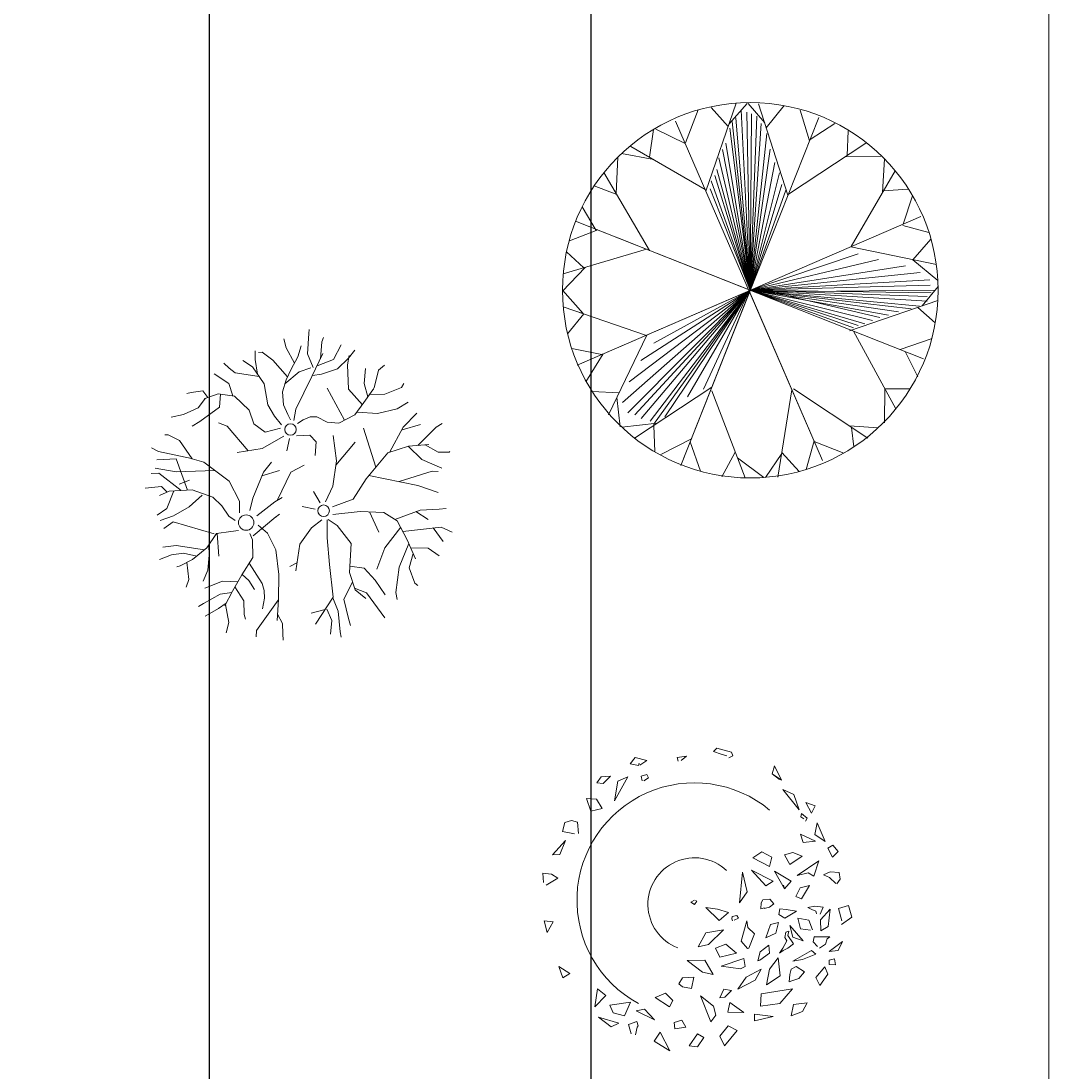
# Model space of a CAD drawing. Units: inches. Extents: x 8049 to 8459, y 820 to 1350.
# Tile 14 of 25: x 8170 to 8197, y 879 to 906. Entities that reach past the tile are written whole.
import ezdxf

# ---------------------------------------------------------------- set-up
doc = ezdxf.new("R2010")
doc.units = ezdxf.units.IN
doc.header["$MEASUREMENT"] = 0
for name, color, linetype, lineweight in [('A-ANNO-DIMS', 2, 'Continuous', 18), ('L-PLNT-BEDS', 94, 'Continuous', 18), ('zelen', 69, 'Continuous', 13)]:
    doc.layers.add(name, color=color, linetype=linetype, lineweight=lineweight)
doc.styles.get("Standard").update_dxf_attribs({"font": 'arial.ttf'})
doc.dimstyles.get("Standard").update_dxf_attribs({"dimtxt": 0.18, "dimasz": 0.18, "dimexe": 0.18, "dimexo": 0.0625, "dimgap": 0.09, "dimtad": 0, "dimtih": 1, "dimtoh": 1, "dimdec": 4, "dimzin": 0, "dimdsep": 46, "dimtxsty": 'Standard', "dimcen": 0.09, "dimadec": 0, "dimazin": 0, "dimtfac": 1, "dimtdec": 4, "dimtofl": 0, "dimtmove": 0, "dimatfit": 3, "dimfxl": 1, "dimtolj": 1, "dimtzin": 0, "dimarcsym": 0})

# ---------------------------------------------------------------- blocks, each defined once
blk = doc.blocks.new('T40C')
for p, q in [((-0.1219, 0.4263), (-0.1133, 0.5002)), ((-0.0016, 0.4444), (-0.055, 0.5069)), ((-0.0016, 0.0138), (-0.0016, 0.5115)), ((-0.0016, 0.5115), (-0.0016, -0.4769)), ((-0.0016, 0.4364), (0.0585, 0.5048)), ((0.1041, 0.4402), (0.0754, 0.5038)), ((-0.0047, 0.2984), (-0.1711, 0.4799)), ((-0.0016, 0.2889), (0.1386, 0.4896)), ((0.0979, 0.4313), (0.1806, 0.4751)), ((0.2217, 0.4068), (0.1848, 0.4759)), ((-0.2, 0.2178), (-0.2513, 0.4459)), ((-0.2374, 0.3843), (-0.221, 0.4586)), ((-0.1327, 0.438), (-0.2166, 0.4607)), ((0.2091, 0.2244), (0.2252, 0.4573)), ((-0.0016, 0.0138), (0.1054, 0.4378)), ((-0.0016, 0.0138), (0.1166, 0.4328)), ((0.0011, 0.0164), (0.1417, 0.4349)), ((0.0011, 0.0164), (0.1801, 0.4343)), ((0.0011, 0.0164), (0.161, 0.432)), ((0.2208, 0.3933), (0.2879, 0.4166)), ((-0.3045, 0.3219), (-0.313, 0.3998)), ((-0.2369, 0.3817), (-0.2976, 0.4118)), ((-0.0016, 0.0138), (0.2033, 0.4135)), ((-0.0016, 0.0138), (0.0852, 0.4075)), ((0.2979, 0.3132), (0.3134, 0.399)), ((0.3508, 0.3661), (-0.3487, -0.3333)), ((0.0011, 0.0164), (-0.3443, 0.3618)), ((-0.3443, 0.3618), (0.3464, -0.329)), ((0.0011, 0.0164), (0.3508, 0.3661)), ((-0.0016, 0.0138), (0.2072, 0.3567)), ((0.0011, 0.0164), (0.0491, 0.3369)), ((-0.3055, 0.3229), (-0.3893, 0.3231)), ((0.3008, 0.3162), (0.3801, 0.3306)), ((-0.3838, 0.2523), (-0.4084, 0.2975)), ((-0.0016, 0.0138), (0.1989, 0.2926)), ((0.0011, 0.0164), (0.0175, 0.3021)), ((0.3847, 0.2335), (0.4047, 0.2984)), ((-0.377, 0.2509), (-0.4492, 0.2275)), ((-0.2034, 0.2144), (-0.4335, 0.2627)), ((-0.0016, 0.0138), (0.1836, 0.2378)), ((0.2092, 0.2254), (0.4418, 0.2362)), ((0.3861, 0.2336), (0.4597, 0.1963)), ((0.3915, 0.2339), (0.3982, 0.2342)), ((-0.4278, 0.1246), (-0.4601, 0.209)), ((0.4263, 0.1181), (0.4586, 0.1989)), ((-0.2946, 0.0138), (-0.4744, 0.1635)), ((0.2937, 0.0138), (0.4738, 0.1555)), ((-0.4281, 0.1249), (-0.4899, 0.1006)), ((0.4291, 0.1204), (0.4873, 0.0978)), ((-0.4418, 0.0138), (-0.4967, 0.0634)), ((0.4315, 0.0138), (0.491, 0.0679)), ((-0.4277, 0.0138), (-0.4952, -0.0443)), ((0.4953, 0.0138), (-0.4939, 0.0138)), ((-0.2846, 0.0167), (-0.4721, -0.1432)), ((-0.0016, 0.0138), (-0.4477, -0.1559)), ((-0.0016, 0.0138), (-0.4464, -0.1312)), ((-0.0016, 0.0138), (-0.4422, -0.1429)), ((-0.0016, 0.0138), (-0.4379, -0.1735)), ((-0.0016, 0.0138), (-0.4328, -0.1117)), ((-0.0016, 0.0138), (-0.4324, -0.1862)), ((-0.4324, -0.1862), (-0.0016, 0.0138)), ((-0.0016, 0.0138), (-0.4146, -0.0968)), ((-0.0016, 0.0138), (-0.4013, -0.1946)), ((-0.0016, 0.0138), (-0.3864, -0.0775)), ((-0.0016, 0.0138), (-0.3647, -0.0593)), ((-0.0016, 0.0138), (-0.3588, -0.1967)), ((-0.0016, 0.0138), (-0.3309, -0.0302)), ((-0.0016, 0.0138), (-0.3156, -0.0151)), ((-0.0016, 0.0138), (-0.3007, -0.0042)), ((-0.0016, 0.0138), (-0.2917, 0.0059)), ((-0.0016, 0.0138), (-0.2861, -0.1863)), ((-0.0016, 0.0138), (-0.2311, -0.181)), ((-0.0016, 0.0138), (-0.0528, -0.0021)), ((-0.0016, 0.0138), (-0.0528, -0.0021)), ((-0.0016, 0.0138), (0.0011, 0.0164)), ((-0.0016, 0.0138), (0.4953, 0.0138)), ((-0.0016, 0.0138), (0.0088, -0.2669)), ((-0.0016, 0.0138), (0.0243, -0.2768)), ((-0.0016, 0.0138), (0.0408, -0.3033)), ((-0.0016, 0.0138), (0.0625, -0.3241)), ((-0.0016, 0.0138), (0.0872, -0.3518)), ((-0.0016, 0.0138), (0.1104, -0.3878)), ((-0.0016, 0.0138), (0.1339, -0.4064)), ((-0.0016, 0.0138), (0.1521, -0.4202)), ((-0.0016, 0.0138), (0.1669, -0.4211)), ((-0.0016, 0.0138), (0.1801, -0.4202)), ((-0.0016, 0.0138), (0.1959, -0.4202)), ((-0.0016, 0.0138), (0.2013, -0.3955)), ((-0.0016, 0.0138), (0.2072, -0.3832)), ((-0.0016, 0.0138), (0.2062, -0.3647)), ((-0.0016, 0.0138), (0.2018, -0.3233)), ((-0.0016, 0.0138), (0.2038, -0.3052)), ((-0.0016, 0.0138), (0.2044, -0.2809)), ((-0.0016, 0.0138), (0.1983, -0.2504)), ((-0.0016, 0.0138), (0.197, -0.2334)), ((-0.0016, 0.0138), (0.2007, -0.2173)), ((-0.0016, 0.0138), (0.1959, -0.1959)), ((0.285, 0.0138), (0.4722, -0.133)), ((0.2917, 0.0138), (0.3747, 0.0138)), ((0.4349, 0.0169), (0.4927, -0.0276)), ((-0.0528, -0.0021), (-0.4551, -0.1664)), ((-0.0528, -0.0021), (-0.3463, -0.045)), ((-0.4294, -0.1068), (-0.4874, -0.0863)), ((0.4191, -0.0914), (0.4833, -0.0909)), ((0.4217, -0.0934), (0.4533, -0.184)), ((-0.4387, -0.1147), (-0.459, -0.1779)), ((-0.3712, -0.2192), (-0.4529, -0.1923)), ((-0.2066, -0.1906), (-0.4335, -0.23)), ((-0.2067, -0.1914), (-0.2414, -0.4204)), ((0.2042, -0.1867), (0.2149, -0.4325)), ((0.2071, -0.1897), (0.4318, -0.2236)), ((-0.3712, -0.2192), (-0.3953, -0.2872)), ((0.3628, -0.2132), (0.4476, -0.1967)), ((0.3755, -0.2151), (0.3928, -0.2871)), ((-0.0016, -0.2596), (-0.1424, -0.4599)), ((-0.0016, -0.2565), (0.16, -0.4525)), ((-0.3126, -0.2938), (-0.3837, -0.3016)), ((-0.3124, -0.2971), (-0.3082, -0.3761)), ((0.3007, -0.2833), (0.3874, -0.2905)), ((0.3008, -0.2851), (0.3017, -0.3787)), ((-0.2322, -0.3601), (-0.2902, -0.3882)), ((-0.2315, -0.3548), (-0.2033, -0.4394)), ((0.2123, -0.3741), (0.1875, -0.442)), ((0.212, -0.3667), (0.2724, -0.3967)), ((-0.1046, -0.4061), (-0.1917, -0.4425)), ((-0.1086, -0.4118), (-0.0869, -0.4727)), ((-0.0016, -0.4144), (-0.047, -0.4779)), ((-0.0016, -0.4109), (0.0515, -0.477)), ((0.1172, -0.4006), (0.0947, -0.4728)), ((0.1259, -0.4112), (0.1857, -0.4428))]:
    blk.add_line(p, q)
blk.add_circle((-0.0016, 0.0138), 0.496)
blk = doc.blocks.new('z_115')
for p, q in [((-18.8, 436.5), (-14.5, 500.6)), ((-14.5, 500.6), (-13.6, 513.4)), ((-86.5, 455.8), (-94.6, 483.9)), ((22, 420.7), (26.8, 474.3)), ((26.8, 474.3), (31.7, 488.4)), ((-184.5, 418.6), (-185.4, 446.1)), ((-162.6, 441.7), (-174.6, 440.4)), ((-129.1, 416.7), (-162.6, 441.7)), ((-60.7, 407), (-86.5, 455.8)), ((-49.9, 426.9), (-39.4, 462.2)), ((-1.4, 393.4), (-18.8, 436.5)), ((-4.9, 364.2), (29.9, 437.2)), ((63.4, 418.3), (87.8, 464.7)), ((111.2, 422.4), (130.6, 448.1)), ((-267.7, 390.7), (-284, 406.4)), ((-193.4, 394.9), (-223.9, 415.7)), ((-177.4, 372), (-184.5, 418.6)), ((-82.4, 363.5), (-129.1, 416.7)), ((-71.1, 387.5), (-49.9, 426.9)), ((11.4, 398.3), (63.4, 418.3)), ((76.1, 388.5), (111.2, 422.4)), ((107.5, 401.6), (113, 430.8)), ((111.2, 324.1), (107.5, 401.6)), ((205.4, 384.6), (225.1, 401)), ((-268.3, 342.4), (-315.1, 373.1)), ((-248.2, 376.3), (-267.7, 390.7)), ((-172.4, 364.7), (-248.2, 376.3)), ((-156.2, 341.4), (-193.4, 394.9)), ((-90.7, 340.9), (-45.9, 379.2)), ((-86.9, 353.9), (-71.1, 387.5)), ((-45.9, 379.2), (-8.3, 392.3)), ((-3.1, 368.1), (25.6, 372.2)), ((25.6, 372.2), (76.1, 388.5)), ((160.2, 342.1), (164.2, 389.5)), ((192.5, 328.6), (205.4, 384.6)), ((-255.3, 302.8), (-268.3, 342.4)), ((-144.5, 275.1), (-156.2, 341.4)), ((-98.3, 315.8), (-86.9, 353.9)), ((-55.7, 261), (-4.9, 364.2)), ((171.8, 299.6), (160.2, 342.1)), ((278.7, 329.2), (286.1, 342.4)), ((-387.5, 313.5), (-401, 310.3)), ((-350.5, 319.6), (-387.5, 313.5)), ((-335.4, 298.2), (-350.5, 319.6)), ((-302.1, 309.7), (-346.5, 294.3)), ((-250.4, 302), (-302.1, 309.7)), ((-294.4, 308.5), (-298.1, 267.8)), ((-203.9, 258.1), (-250.4, 302)), ((-95.5, 274.5), (-98.3, 315.8)), ((97.9, 225.7), (42.8, 327.6)), ((155.1, 275.2), (111.2, 324.1)), ((159.9, 282.2), (182.3, 314.8)), ((177.4, 307.7), (226.4, 308.4)), ((182.3, 314.8), (191.3, 327)), ((226.4, 308.4), (278.7, 329.2)), ((-342.4, 295.8), (-365.9, 265.5)), ((-298.1, 267.8), (-360.4, 221.6)), ((-124.1, 238.9), (-144.5, 275.1)), ((-81.6, 243.7), (-95.5, 274.5)), ((131.2, 242.8), (159.9, 282.2)), ((264.6, 262), (300, 283.1)), ((-412.1, 244), (-450.9, 235.7)), ((-365.9, 265.5), (-412.1, 244)), ((-189.7, 214.3), (-203.9, 258.1)), ((-101.3, 211.6), (-124.1, 238.9)), ((-72.6, 227.6), (-81.6, 243.7)), ((-61.9, 224.8), (-55.7, 261)), ((-33, 226.8), (-11.1, 237)), ((-11.1, 237), (10.2, 237)), ((10.2, 237), (43.7, 220)), ((80.7, 216.8), (131.2, 242.8)), ((137.8, 251.8), (202.7, 247.6)), ((202.7, 247.6), (264.6, 262)), ((284, 204.3), (327.4, 248.5)), ((-360.4, 221.6), (-384.1, 206.6)), ((-273.2, 207.5), (-301.5, 217.8)), ((-206.8, 129.4), (-273.2, 207.5)), ((-152.8, 187.7), (-189.7, 214.3)), ((-104.5, 200.6), (-152.8, 187.7)), ((-50.6, 215.3), (-33, 226.8)), ((43.7, 220), (80.7, 216.8)), ((197.6, 76.9), (158.9, 201.1)), ((241, 124.1), (284, 204.3)), ((281.2, 196), (338.5, 212.3)), ((330.6, 146), (388.4, 203.7)), ((388.4, 203.7), (407.5, 215.5)), ((-461.1, 179.4), (-470.9, 180)), ((-424.4, 162.1), (-461.1, 179.4)), ((-94.2, 175.3), (-163.2, 136.1)), ((-75.7, 168.1), (-84.7, 128.4)), ((-53.8, 176.8), (-11.4, 178.7)), ((-11.4, 178.7), (8, 157.9)), ((73, 96.7), (62.2, 177.8)), ((-491.6, 126.5), (-513.4, 138)), ((-384.4, 104), (-424.4, 162.1)), ((-163.2, 136.1), (-242.4, 123.9)), ((8, 157.9), (5.5, 114)), ((71.1, 83.3), (132.4, 156.9)), ((235.6, 122.3), (301.5, 143.8)), ((299.9, 143.7), (343.1, 101.2)), ((301.5, 143.8), (365.3, 148.6)), ((354.1, 147.8), (394.5, 124.9)), ((-435.2, 103.8), (-496.2, 99.9)), ((-387.1, 104.7), (-491.6, 126.5)), ((-399.6, 4.6), (-435.2, 103.8)), ((-347.4, 93.2), (-391.5, 106)), ((166.9, 40.4), (235.6, 122.3)), ((343.1, 101.2), (406.3, 74)), ((394.5, 124.9), (429.4, 124.9)), ((429.4, 124.9), (432.1, 126.5)), ((-434.9, 62.5), (-501.7, 74)), ((-312.8, 66.9), (-434.9, 62.5)), ((-267.7, 32.7), (-347.4, 93.2)), ((-158.6, 61.2), (-132.7, 93.2)), ((-71.8, 61.2), (-29.6, 83.9)), ((61.6, 17), (73, 96.7)), ((-490, 58), (-515, 57)), ((-419.6, 3.5), (-490, 58)), ((-392.7, 35.9), (-425.7, 23.1)), ((-192.8, -21.5), (-158.6, 61.2)), ((-163.3, 49.8), (-107.5, 66.3)), ((-115.7, -28.8), (-71.8, 61.2)), ((126, -24.3), (166.9, 40.4)), ((175.7, 50.8), (330.2, 19.2)), ((271, 31.3), (376.4, 64.1)), ((376.4, 64.1), (395.5, 63.1)), ((-481.7, 16.3), (-533.5, 10.6)), ((-457.4, 1.3), (-488.2, -12.8)), ((-464, -1.8), (-481.7, 16.3)), ((-442.9, 2.1), (-465.1, -53.8)), ((-385, 5.4), (-457.4, 1.3)), ((-319.1, -17.9), (-385, 5.4)), ((-235, -30.4), (-267.7, 32.7)), ((20.8, -35.8), (0, 0)), ((38.1, -32.9), (61.6, 17)), ((330.2, 19.2), (395.5, -3.5)), ((-353.3, -11.5), (-394.5, -49)), ((-290.4, -45.2), (-319.1, -17.9)), ((-234.8, -67.7), (-235, -30.4)), ((-201.7, -60.6), (-192.8, -21.5)), ((-179.5, -77.2), (-122.3, -32.7)), ((-122.3, -32.7), (-99.2, -18.9)), ((60.5, -49.2), (126, -24.3)), ((-465.1, -53.8), (-495.6, -74.6)), ((-394.5, -49), (-444.1, -77.2)), ((-268, -78.8), (-290.4, -45.2)), ((5.5, -56.2), (-36, -48)), ((61.1, -73.3), (147.5, -63.4)), ((147.5, -63.4), (222.4, -66.3)), ((177.6, -64.6), (207.3, -129.1)), ((222.4, -66.3), (265.5, -93.5)), ((258.1, -88.8), (337.6, -59.6)), ((324, -63.1), (363.7, -88.7)), ((337.6, -59.6), (397.9, -55.7)), ((397.9, -55.7), (420.7, -53.5)), ((-444.1, -77.2), (-486, -91.9)), ((-444.4, -96.7), (-474, -117.5)), ((-314.6, -134.2), (-444.4, -96.7)), ((-248.3, -92.1), (-268, -78.8)), ((-119.3, -80.2), (-191.3, -140.3)), ((-108.1, -71.7), (-122, -82.3)), ((25.9, -89.8), (-6.8, -115.6)), ((43, -89.7), (43.4, -146.7)), ((46.4, -88.4), (74.8, -107.6)), ((265.5, -93.5), (296.9, -152.8)), ((-262.1, -127.1), (-307.1, -133.2)), ((-305.3, -133), (-300.3, -204.7)), ((-237.6, -123.2), (-262.1, -127.1)), ((-202.1, -132.9), (-193.1, -153.7)), ((-175.4, -107.1), (-146.3, -132.3)), ((-146.3, -132.3), (-119.5, -185.4)), ((-6.8, -115.6), (-43.1, -167.5)), ((74.8, -107.6), (119.8, -164.9)), ((276.2, -113.6), (225.5, -179)), ((282.9, -126.4), (404.4, -113.1)), ((379.5, -115), (410.6, -158.2)), ((404.4, -113.1), (439.8, -128.7)), ((-307.1, -133.2), (-338.5, -178.7)), ((-193.1, -153.7), (-192.8, -209.8)), ((43.4, -146.7), (50.5, -231.2)), ((119.8, -164.9), (114, -256.5)), ((302.2, -165.1), (271.3, -239.9)), ((296.9, -152.8), (323.1, -213.9)), ((-435.8, -171.7), (-477.7, -176.8)), ((-412.1, -196), (-449.7, -200.8)), ((-345.7, -184.7), (-435.8, -171.7)), ((-370.3, -205.2), (-412.1, -196)), ((-338.5, -178.7), (-383.2, -215.9)), ((-331.8, -169), (-330.2, -201.8)), ((-119.5, -185.4), (-109.6, -262.9)), ((-43.1, -167.5), (-56.4, -251.1)), ((225.5, -179), (200.5, -246.3)), ((315.6, -196.4), (303.1, -242.1)), ((308, -178.8), (363.4, -180)), ((363.4, -180), (398.2, -204)), ((-449.7, -200.8), (-487.6, -215.5)), ((-383.2, -215.9), (-422.9, -235.4)), ((-401, -224.6), (-395.5, -279.3)), ((-330.2, -201.8), (-335.4, -249.2)), ((-192.8, -209.8), (-226.7, -263.9)), ((-203.8, -227.4), (-162.3, -292.1)), ((-52.5, -226.5), (-74.8, -238)), ((50.5, -231.2), (62.2, -335)), ((-422.9, -235.4), (-433, -238.6)), ((-335.4, -249.2), (-349.3, -284.7)), ((-226.7, -263.9), (-257.2, -316.1)), ((-226, -262.8), (-205.1, -282.2)), ((-109.6, -262.9), (-111.5, -342.4)), ((114, -256.5), (131.8, -311.6)), ((115.2, -236.5), (160.5, -243.1)), ((160.5, -243.1), (195.3, -280.9)), ((271.3, -239.9), (260.9, -320.6)), ((303.1, -242.1), (321.2, -290.5)), ((-395.5, -279.3), (-403.2, -303.6)), ((-288.3, -284.4), (-344.7, -307.1)), ((-239.6, -286.1), (-288.3, -284.4)), ((-205.1, -282.2), (-187, -310.7)), ((-162.3, -292.1), (-156.8, -314.2)), ((123.9, -287.2), (95.8, -341.4)), ((195.3, -280.9), (227, -327.3)), ((321.2, -290.5), (330.8, -298.2)), ((-296, -325.4), (-348.3, -355.5)), ((-259.3, -320.1), (-296, -325.4)), ((-257.2, -316.1), (-280.9, -362.2)), ((-249.1, -302.2), (-221.1, -346.5)), ((-156.8, -314.2), (-155.8, -338.2)), ((130.2, -306.7), (167.9, -320.9)), ((131.8, -311.6), (166, -339.5)), ((167.9, -320.9), (225.5, -401)), ((260.9, -320.6), (264.9, -343)), ((-348.3, -355.5), (-364.4, -365.1)), ((-276.6, -353.8), (-301.5, -371.5)), ((-278.8, -358.2), (-268.6, -415.4)), ((-221.1, -346.5), (-219.9, -389.8)), ((-111.6, -344.9), (-180.5, -441.3)), ((-155.8, -338.2), (-161.7, -371.8)), ((-111.5, -342.4), (-115.5, -409.6)), ((62.2, -335), (6.5, -421.2)), ((61.1, -336.8), (77.6, -379.5)), ((95.8, -341.4), (111.2, -402.9)), ((-301.5, -371.5), (-343.7, -395.5)), ((-219.9, -389.8), (-215.6, -404.5)), ((-114.3, -389.5), (-97.9, -418.6)), ((36.7, -374.4), (-8, -385.6)), ((42.5, -373), (58.5, -409.6)), ((77.6, -379.5), (84.1, -444.9)), ((-268.6, -415.4), (-277.2, -447.7)), ((-97.9, -418.6), (-97.3, -451.3)), ((58.5, -409.6), (53.6, -452.5)), ((111.2, -402.9), (117.7, -425.3)), ((-180.5, -441.3), (-181.7, -460.9)), ((-97.3, -451.3), (-96.4, -471.1)), ((84.1, -444.9), (87.2, -462.2))]:
    blk.add_line(p, q)
for centre, radius in [((-73, 196.5), 18.1), ((31.9, -61.1), 18.3), ((-213.5, -98.7), 24.4)]:
    blk.add_circle(centre, radius)
blk = doc.blocks.new('z_66')
for p, q in [((83.2, 488.9), (72.7, 477.7)), ((72.7, 477.7), (96.4, 469.7)), ((129.8, 476.2), (83.2, 488.9)), ((96.4, 469.7), (114.5, 463.9)), ((134, 464.6), (129.8, 476.2)), ((-176.4, 458.5), (-191.7, 438.6)), ((-191.7, 438.6), (-165.6, 433.5)), ((-139.2, 449.4), (-176.4, 458.5)), ((-165.6, 433.5), (-163.6, 441.1)), ((-165.6, 433.5), (-165.6, 433.5)), ((-161.1, 434.6), (-139.2, 449.4)), ((-13.6, 463.6), (-42.5, 459.2)), ((-42.5, 459.2), (-39.3, 446.9)), ((-30.3, 449.4), (-13.6, 463.6)), ((114.5, 463.9), (114.5, 463.9)), ((120.4, 457.8), (134, 464.6)), ((-254, 399.9), (-283.6, 397.7)), ((-272.8, 380.7), (-254, 399.9)), ((-138.9, 404.9), (-156.9, 400.2)), ((-156.9, 400.2), (-153.8, 385.4)), ((-133.3, 394.8), (-138.9, 404.9)), ((265.2, 432.1), (258.2, 407.5)), ((258.2, 407.5), (287.4, 387.2)), ((258.2, 407.5), (281.9, 388.6)), ((287.4, 387.2), (265.2, 432.1)), ((-283.6, 397.7), (-297.2, 378.2)), ((-297.2, 378.2), (-277.7, 376)), ((-277.7, 376), (-272.8, 380.7)), ((-241.9, 321.7), (-199.1, 397.3)), ((-231.4, 383.6), (-241.9, 321.7)), ((-199.1, 397.3), (-231.4, 383.6)), ((-148.6, 384.7), (-133.3, 394.8)), ((281.9, 388.6), (281.9, 388.6)), ((344.2, 293.1), (292, 357.2)), ((292, 357.2), (326.8, 341.2)), ((326.8, 341.2), (344.2, 293.1)), ((-330.3, 328.9), (-298.6, 327.1)), ((-316, 288.8), (-330.3, 328.9)), ((-298.6, 327.1), (-280.8, 297.1)), ((383.1, 281.9), (364.4, 316.3)), ((364.4, 316.3), (394.6, 305.1)), ((394.6, 305.1), (383.1, 281.9)), ((-280.8, 297.1), (-316, 288.8)), ((350.8, 280.8), (348.7, 270.3)), ((348.7, 270.3), (358.8, 264.5)), ((369.2, 266.7), (350.8, 280.8)), ((363.3, 256.6), (369.2, 266.7)), ((-399.2, 252.6), (-405.8, 224)), ((-377.9, 259.1), (-399.2, 252.6)), ((-358.4, 254), (-377.9, 259.1)), ((-356, 217.5), (-358.4, 254)), ((358.8, 264.5), (358.8, 264.5)), ((400.9, 251.9), (393.9, 214.6)), ((426.6, 192.2), (400.9, 251.9)), ((-405.8, 224), (-368.2, 216.4)), ((-368.2, 216.4), (-368.2, 216.4)), ((348, 215.7), (356, 188.9)), ((395.3, 193.2), (348, 215.7)), ((393.9, 214.6), (426.6, 192.2)), ((-396.4, 196.1), (-438.1, 150.2)), ((-414.8, 150.9), (-396.4, 196.1)), ((356, 188.9), (395.3, 193.2)), ((450, 180.6), (434.3, 171.2)), ((434.3, 171.2), (449.6, 142.6)), ((467.7, 160.3), (450, 180.6)), ((-438.1, 150.2), (-414.8, 150.9)), ((225.2, 159.9), (197, 140.8)), ((197, 140.8), (249.5, 113.6)), ((256.8, 142.6), (225.2, 159.9)), ((249.5, 113.6), (256.8, 142.6)), ((323.6, 157.8), (297.5, 149.8)), ((297.5, 149.8), (314.6, 119.4)), ((314.6, 119.4), (352.9, 145.5)), ((352.9, 145.5), (323.6, 157.8)), ((449.6, 142.6), (467.7, 160.3)), ((193.1, 101.3), (238, 52.1)), ((261.7, 66.6), (193.1, 101.3)), ((336.9, 84.3), (405.8, 131.7)), ((405.8, 131.7), (389.8, 82.1)), ((-468.4, 91.6), (-466.3, 62.6)), ((-441.6, 89), (-468.4, 91.6)), ((-458.3, 53.9), (-421.1, 76)), ((-421.1, 76), (-441.6, 89)), ((164.3, 94.8), (154.2, -2.2)), ((178.9, 33.3), (164.3, 94.8)), ((265.2, 98.8), (297.2, 42.7)), ((318.8, 66.2), (265.2, 98.8)), ((372.7, 93), (336.9, 84.3)), ((389.8, 82.1), (372.7, 93)), ((441.6, 95.9), (420.7, 86.5)), ((420.7, 86.5), (440.2, 78.5)), ((440.2, 78.5), (459.7, 59.7)), ((470.5, 93.7), (441.6, 95.9)), ((463.2, 57.9), (474, 73.5)), ((474, 73.5), (470.5, 93.7)), ((-466.3, 62.6), (-466.3, 62.6)), ((238, 52.1), (261.7, 66.6)), ((297.2, 42.7), (294.1, 53.6)), ((297.2, 42.7), (318.8, 66.2)), ((347.3, 45.2), (332.7, 18.1)), ((376.9, 52.5), (347.3, 45.2)), ((350.8, 10.9), (376.9, 52.5)), ((459.7, 59.7), (459.7, 59.7)), ((11.8, 6.2), (0, 0)), ((0, 0), (12.2, -6.9)), ((12.2, -6.9), (19.1, 2.9)), ((19.1, 2.9), (15.7, 5.8)), ((154.2, -2.2), (178.9, 33.3)), ((229, 7.2), (223.1, -2.5)), ((250.6, 9.8), (229, 7.2)), ((263.4, -5.4), (250.6, 9.8)), ((332.7, 18.1), (350.8, 10.9)), ((84.6, -21.7), (48, -17)), ((48, -17), (90.1, -58.3)), ((119.4, -32.9), (84.6, -21.7)), ((90.1, -58.3), (119.4, -32.9)), ((223.1, -2.5), (222.7, -20.6)), ((222.7, -20.6), (234.2, -18.1)), ((233.2, -19.9), (249.9, -15.9)), ((234.2, -18.1), (234.2, -18.1)), ((249.9, -15.9), (263.4, -5.4)), ((282.9, -21.3), (279.1, -39.1)), ((302.1, -22.8), (282.9, -21.3)), ((298.6, -50.3), (335.8, -28.6)), ((335.8, -28.6), (302.1, -22.8)), ((393.6, -13), (371, -17)), ((371, -17), (383.5, -23.5)), ((383.5, -23.5), (396.7, -28.9)), ((420, -15.9), (393.6, -13)), ((396.7, -28.9), (398.5, -35.5)), ((410.3, -38), (420, -15.9)), ((442, -22.4), (411.3, -55.4)), ((436, -77.1), (442, -22.4)), ((499.7, -10.9), (468.8, -19.9)), ((468.8, -19.9), (478.8, -58.6)), ((510.9, -47), (499.7, -10.9)), ((-464.2, -59.3), (-436.4, -62.6)), ((-454.5, -96.3), (-464.2, -59.3)), ((-436.4, -62.6), (-454.5, -96.3)), ((131.9, -44.9), (130.2, -52.5)), ((130.2, -52.5), (132.9, -59.3)), ((146.5, -42.3), (131.9, -44.9)), ((138.2, -56.8), (151, -51)), ((151, -51), (146.5, -42.3)), ((177.8, -59), (160.1, -123.8)), ((181, -80.3), (177.8, -59)), ((278.4, -64), (252.6, -70.9)), ((269.7, -98.4), (278.4, -64)), ((279.1, -39.1), (298.6, -50.3)), ((339, -51), (347.7, -84.3)), ((374.1, -56.8), (339, -51)), ((386.3, -87.9), (374.1, -56.8)), ((398.5, -35.5), (399.5, -35.8)), ((411.3, -55.4), (412.7, -90.8)), ((477.5, -70.2), (510.9, -47)), ((478.8, -58.6), (478.8, -58.6)), ((47.7, -96.6), (24, -141.9)), ((104.1, -87.9), (47.7, -96.6)), ((56, -133.9), (104.1, -87.9)), ((202.2, -100.6), (181, -80.3)), ((252.6, -70.9), (237.7, -112.9)), ((237.7, -112.9), (269.7, -98.4)), ((301.7, -95.5), (297.9, -112.2)), ((310.8, -91.9), (301.7, -95.5)), ((307.6, -106), (310.8, -91.9)), ((314.2, -74.2), (356.7, -123)), ((323.3, -111.1), (314.2, -74.2)), ((347.7, -84.3), (379.7, -88.3)), ((379.7, -88.3), (379.7, -88.3)), ((412.7, -90.8), (436, -77.1)), ((111.4, -132.8), (78.3, -146.2)), ((145.1, -162.1), (111.4, -132.8)), ((160.1, -123.8), (179.6, -146.6)), ((183.7, -145.5), (202.2, -100.6)), ((304.5, -123), (291.6, -145.8)), ((297.9, -112.2), (304.5, -123)), ((325.4, -132.4), (307.6, -106)), ((308.3, -145.8), (325.4, -132.4)), ((356.7, -123), (323.3, -111.1)), ((356.7, -123), (356.7, -123)), ((356.7, -123), (356.7, -123)), ((391.2, -110), (388.4, -125.6)), ((388.4, -125.6), (402.3, -140.8)), ((391.2, -110), (393.2, -108.6)), ((441.3, -110), (391.2, -110)), ((427, -133.5), (432.9, -115.8)), ((432.9, -115.8), (441.3, -110)), ((480.9, -124.5), (439.2, -156)), ((467.7, -153.4), (480.9, -124.5)), ((24, -141.9), (56, -133.9)), ((78.3, -146.2), (92.2, -174.1)), ((92.2, -174.1), (145.1, -162.1)), ((179.6, -146.6), (183.7, -145.5)), ((220.6, -157), (212.6, -186)), ((219.2, -183.5), (249.2, -162.1)), ((247.1, -135.7), (220.6, -157)), ((249.2, -162.1), (247.1, -135.7)), ((291.6, -145.8), (281.2, -161.8)), ((281.2, -161.8), (293, -152.7)), ((293, -152.7), (308.3, -145.8)), ((382.5, -152.7), (323.3, -187.4)), ((353.9, -182), (396.7, -164.3)), ((396.7, -164.3), (382.5, -152.7)), ((402.3, -140.8), (402.3, -140.8)), ((407.9, -145.5), (427, -133.5)), ((439.2, -156), (467.7, -153.4)), ((44.5, -184.2), (-10.8, -184.9)), ((-10.8, -184.9), (36.9, -222.2)), ((71, -229.1), (44.5, -184.2)), ((168.1, -178.4), (96.7, -202.6)), ((173, -203.4), (168.1, -178.4)), ((212.6, -186), (219.2, -183.5)), ((277.4, -176.2), (250.2, -212.4)), ((283.3, -233.8), (277.4, -176.2)), ((323.3, -187.4), (353.9, -182)), ((438.5, -183.8), (456.2, -179.1)), ((438.5, -197.6), (438.5, -183.8)), ((458.7, -199), (438.5, -197.6)), ((456.2, -179.1), (458.7, -199)), ((-417.9, -204.1), (-405.1, -239.6)), ((-382.8, -226.5), (-417.9, -204.1)), ((-405.1, -239.6), (-382.8, -226.5)), ((36.9, -222.2), (71, -229.1)), ((96.7, -202.6), (157.6, -211.3)), ((157.6, -211.3), (173, -203.4)), ((223.8, -212.4), (175.4, -237.7)), ((204.3, -246.8), (223.8, -212.4)), ((250.2, -212.4), (240.1, -262.4)), ((314.6, -228.7), (311.8, -252.6)), ((318.4, -212.1), (314.6, -228.7)), ((334.1, -203.7), (318.4, -212.1)), ((360.2, -221.1), (334.1, -203.7)), ((342.8, -241.4), (360.2, -221.1)), ((425.3, -204.5), (396.7, -238.5)), ((409.2, -264.2), (434.3, -228)), ((434.3, -228), (425.3, -204.5)), ((-26.4, -240.3), (-37.6, -258.4)), ((-37.6, -258.4), (-25.8, -268.5)), ((10.1, -237.7), (-26.4, -240.3)), ((2.4, -273.2), (10.1, -237.7)), ((175.4, -237.7), (149.6, -276.1)), ((149.6, -276.1), (204.3, -246.8)), ((240.1, -262.4), (283.3, -233.8)), ((311.8, -252.6), (320.5, -249.3)), ((320.5, -249.3), (342.8, -241.4)), ((396.7, -238.5), (409.2, -264.2)), ((-295.1, -275), (-304.2, -331.5)), ((-304.2, -331.5), (-269, -296)), ((-269, -296), (-295.1, -275)), ((-80, -288), (-112.4, -302.5)), ((-56.7, -311.6), (-80, -288)), ((-25.8, -268.5), (2.4, -273.2)), ((-25.8, -268.5), (-25.8, -268.5)), ((-25.8, -268.5), (-25.8, -268.5)), ((30.6, -297.1), (72.7, -329.3)), ((64, -379.6), (30.6, -297.1)), ((105.1, -276.1), (91.9, -303.6)), ((128.8, -280.4), (105.1, -276.1)), ((108.6, -301.4), (128.8, -280.4)), ((223.8, -290.2), (221.3, -330)), ((322.2, -275), (223.8, -290.2)), ((282.2, -321.7), (322.2, -275)), ((-191.1, -317.4), (-256.8, -326.4)), ((-256.8, -326.4), (-245.7, -350.3)), ((-209.8, -360.4), (-191.1, -317.4)), ((-112.4, -302.5), (-67.5, -331.8)), ((-67.5, -331.8), (-56.7, -311.6)), ((72.7, -329.3), (79.3, -357.9)), ((91.9, -303.6), (108.6, -301.4)), ((117.3, -348.8), (124.2, -317.7)), ((124.2, -317.7), (168.8, -349.9)), ((221.3, -330), (282.2, -321.7)), ((325.7, -323.9), (318.4, -360.1)), ((368.9, -319.2), (325.7, -323.9)), ((354.3, -346.3), (368.9, -319.2)), ((-292, -364.4), (-252, -395.5)), ((-228.3, -383.9), (-292, -364.4)), ((-245.7, -350.3), (-209.8, -360.4)), ((-172.6, -344.9), (-146.9, -338.7)), ((-114.8, -372.7), (-172.6, -344.9)), ((-146.9, -338.7), (-114.8, -372.7)), ((79.3, -357.9), (64, -379.6)), ((168.8, -349.9), (117.3, -348.8)), ((201.8, -355), (202.2, -376.3)), ((261, -362.2), (201.8, -355)), ((202.2, -376.3), (261, -362.2)), ((318.4, -360.1), (354.3, -346.3)), ((-252, -395.5), (-228.3, -383.9)), ((-197.3, -388.3), (-171.2, -377.8)), ((-188.3, -416.9), (-197.3, -388.3)), ((-169.5, -396.6), (-174.7, -420.5)), ((-171.2, -377.8), (-166, -391.5)), ((-166, -391.5), (-169.5, -396.6)), ((-27.8, -374.5), (-52.9, -381.8)), ((-52.9, -381.8), (-50.8, -402)), ((-50.8, -402), (-15.3, -396.2)), ((-15.3, -396.2), (-27.8, -374.5)), ((91.9, -424.8), (119, -391.5)), ((119, -391.5), (146.9, -406.4)), ((-174.7, -420.5), (-174.7, -420.5)), ((-116.2, -441.1), (-96.4, -411.8)), ((-96.4, -411.8), (-65.8, -470.8)), ((21.6, -417.2), (-4.5, -455.6)), ((42.1, -428.8), (21.6, -417.2)), ((21.6, -458.1), (42.1, -428.8)), ((106.8, -455.6), (91.9, -424.8)), ((146.9, -406.4), (106.8, -455.6)), ((-65.8, -470.8), (-116.2, -441.1)), ((-4.5, -455.6), (21.6, -458.1))]:
    blk.add_line(p, q)
for centre, radius, start, end in [((11.8, 6.2), 372.3, 50.2118, 241.5185), ((12.2, -6.9), 147.8, 46.7611, 248.9067)]:
    blk.add_arc(centre, radius, start, end)
blk = doc.blocks.new('*D58')
at = {"layer": 'A-ANNO-DIMS', "color": 0, "lineweight": -2, "transparency": 16777216}
for p, q in [((8139.397, 1162.808), (8139.397, 820.091)), ((8175.397, 1162.808), (8175.397, 820.091)), ((8139.577, 820.271), (8157.179, 820.271)), ((8175.217, 820.271), (8157.616, 820.271))]:
    blk.add_line(p, q, dxfattribs=at)
at = {"layer": 'A-ANNO-DIMS', "color": 0, "transparency": 16777216}
for points in [[(8139.577, 820.301), (8139.577, 820.241), (8139.397, 820.271)], [(8175.217, 820.301), (8175.217, 820.241), (8175.397, 820.271)]]:
    blk.add_solid(points, dxfattribs=at)
at = {"layer": 'Defpoints', "color": 0, "transparency": 16777216}
for p in [(8139.397, 1162.871), (8175.397, 1162.871), (8175.397, 820.271)]:
    blk.add_point(p, dxfattribs=at)
at = {"layer": 'A-ANNO-DIMS', "color": 0, "transparency": 16777216, "insert": (8157.397, 820.271), "char_height": 0.18, "attachment_point": 5}
blk.add_mtext('\\A1;36', dxfattribs=at)
blk = doc.blocks.new('*D71')
at = {"layer": 'A-ANNO-DIMS', "color": 0, "lineweight": -2, "transparency": 16777216}
for p, q in [((8185.397, 1045.808), (8185.397, 820.091)), ((8239.397, 1045.808), (8239.397, 820.091)), ((8185.577, 820.271), (8212.179, 820.271)), ((8239.217, 820.271), (8212.616, 820.271))]:
    blk.add_line(p, q, dxfattribs=at)
at = {"layer": 'A-ANNO-DIMS', "color": 0, "transparency": 16777216}
for points in [[(8185.577, 820.301), (8185.577, 820.241), (8185.397, 820.271)], [(8239.217, 820.301), (8239.217, 820.241), (8239.397, 820.271)]]:
    blk.add_solid(points, dxfattribs=at)
at = {"layer": 'Defpoints', "color": 0, "transparency": 16777216}
for p in [(8185.397, 1045.871), (8239.397, 1045.871), (8239.397, 820.271)]:
    blk.add_point(p, dxfattribs=at)
at = {"layer": 'A-ANNO-DIMS', "color": 0, "transparency": 16777216, "insert": (8212.397, 820.271), "char_height": 0.18, "attachment_point": 5}
blk.add_mtext('\\A1;54', dxfattribs=at)
blk = doc.blocks.new('*D76')
at = {"layer": 'A-ANNO-DIMS', "color": 0, "lineweight": -2, "transparency": 16777216}
for p, q in [((8083.397, 1054.808), (8083.397, 820.091)), ((8299.397, 1054.808), (8299.397, 820.091)), ((8083.577, 820.271), (8191.107, 820.271)), ((8299.217, 820.271), (8191.688, 820.271))]:
    blk.add_line(p, q, dxfattribs=at)
at = {"layer": 'A-ANNO-DIMS', "color": 0, "transparency": 16777216}
for points in [[(8083.577, 820.301), (8083.577, 820.241), (8083.397, 820.271)], [(8299.217, 820.301), (8299.217, 820.241), (8299.397, 820.271)]]:
    blk.add_solid(points, dxfattribs=at)
at = {"layer": 'Defpoints', "color": 0, "transparency": 16777216}
for p in [(8083.397, 1054.871), (8299.397, 1054.871), (8299.397, 820.271)]:
    blk.add_point(p, dxfattribs=at)
at = {"layer": 'A-ANNO-DIMS', "color": 0, "transparency": 16777216, "insert": (8191.397, 820.271), "char_height": 0.18, "attachment_point": 5}
blk.add_mtext('\\A1;216', dxfattribs=at)

msp = doc.modelspace()

# ---------------------------------------------------------------- linework, layer by layer
at = {"layer": 'L-PLNT-BEDS'}
msp.add_line((8197.3974, 949.8706), (8197.3974, 853.8706), dxfattribs=at)

# ---------------------------------------------------------------- block references
at = {"layer": 'zelen', "xscale": 9.920223989974332, "yscale": 9.920223989974332, "zscale": 9.920223989974332, "rotation": 158.4000000000004}
msp.add_blockref('T40C', (8189.6083, 899.3535), dxfattribs=at)
at = {"layer": 'zelen', "xscale": 0.0082668533249786, "yscale": 0.0082668533249786, "zscale": 0.0082668533249786}
for name, p in [('z_115', (8178.1293, 893.9457)), ('z_66', (8188.0109, 883.179))]:
    msp.add_blockref(name, p, dxfattribs=at)

# ---------------------------------------------------------------- dimensions: what is measured, and where the dimension line sits
at = {"layer": 'A-ANNO-DIMS'}
for base, p1, p2, picture, middle in [((8175.3974, 820.2706), (8139.3974, 1162.8706), (8175.3974, 1162.8706), '*D58', (8157.3974, 820.2706)), ((8299.3974, 820.2706), (8083.3974, 1054.8706), (8299.3974, 1054.8706), '*D76', (8191.3974, 820.2706)), ((8239.3974, 820.2706), (8185.3974, 1045.8706), (8239.3974, 1045.8706), '*D71', (8212.3974, 820.2706))]:
    dim = msp.add_linear_dim(base=base, p1=p1, p2=p2, dimstyle='Standard', override={"dimdec": 0, "dimlfac": 1, "dimrnd": 0, "dimzin": 0, "dimdsep": 46, "dimlunit": 2}, dxfattribs=at)
    dim.commit()
    dim.dimension.update_dxf_attribs({"geometry": picture, "text_midpoint": middle})

doc.saveas('drawing.dxf')
